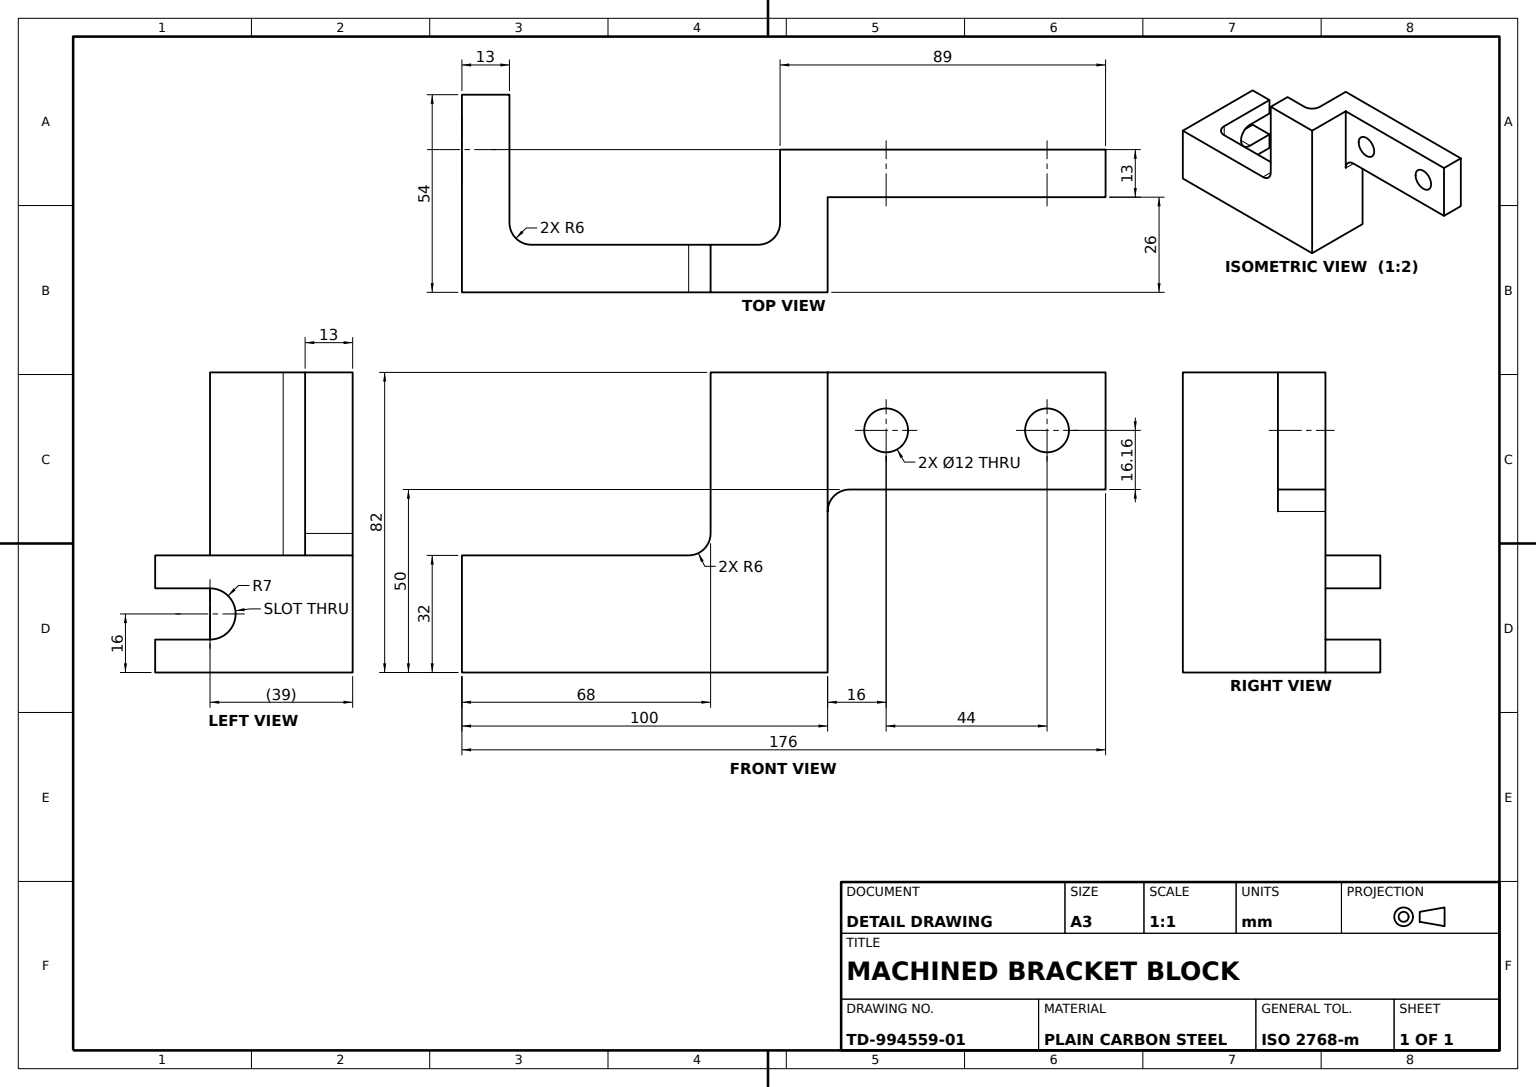
SolidWorks part; units mm, degrees
material "Plain Carbon Steel"
ref_plane "Front Plane" through (0, 0, 0) normal (0, 0, 1) x (1, 0, 0)
ref_plane "Top Plane" through (0, 0, 0) normal (0, 1, 0) x (1, 0, 0)
ref_plane "Right Plane" through (0, 0, 0) normal (1, 0, 0) x (0, 0, -1)
sketch "Base Profile Sketch" plane through (0, 0, 0) normal (0, 0, 1) x (1, 0, 0)
  line L0 (0, 0) -> (100, 0)
  line L1 (100, 0) -> (100, 82)
  line L2 (100, 82) -> (68, 82)
  line L3 (68, 82) -> (68, 38)
  line L4 (62, 32) -> (0, 32)
  line L5 (0, 32) -> (0, 0)
  arc A0 (62, 32) -> (68, 38) centre (62, 38) ccw
  dimension "D1" = 6
  dimension "D2" = 68
  dimension "D3" = 100
  dimension "D4" = 82
extrude "Base Profile 13mm" add sketch "Base Profile Sketch" along normal blind 13
sketch "Upright Block Sketch" plane through (0, 0, 0) normal (0, -1, 0) x (1, 0, 0)
  line L0 (0, 0) -> (0, -54)
  line L1 (0, -54) -> (13, -54)
  line L2 (13, -54) -> (13, -6)
  line L3 (0, 0) -> (100, 0) construction
  line L5 (87, -6) -> (87, -26)
  line L6 (87, -26) -> (100, -26)
  line L7 (100, -26) -> (100, 0)
  line L8 (19, 0) -> (81, 0)
  line L9 (0, 0) -> (100, 0)
  line L10 (100, 13) -> (100, 0) construction
  arc A0 (19, 0) -> (13, -6) centre (19, -6) ccw
  arc A1 (81, 0) -> (87, -6) centre (81, -6) cw
  point P14 (13, 0)
  line M1 (0, 0) -> (100, 0)
  dimension "D1" = 6
  dimension "D2" = 6
  dimension "D3" = 13
  dimension "D4" = 26
  dimension "D5" = 54
extrude "Upright Block 82mm" add sketch "Upright Block Sketch" against normal blind 82 contours A0 L0 L1 L2 M1 | A1 L5 L6 L7 M1
sketch "Rectangular Cut Sketch" plane through (0, 0, 0) normal (-1, 0, 0) x (0, 0, 1)
  line L0 (-54, 82) -> (0, 82)
  line L1 (0, 82) -> (0, 32)
  line L2 (0, 38) -> (0, 32) construction
  line L3 (0, 82) -> (0, 32) construction
  line L4 (0, 32) -> (-54, 32)
  line L5 (-54, 82) -> (-54, 0) construction
  line L6 (-54, 32) -> (-54, 82)
  dimension "D1" = 50
extrude "Rectangular Cut 20mm" cut sketch "Rectangular Cut Sketch" against normal blind 20
sketch "Pocket Cut Sketch" plane through (0, 0, -54) normal (0, 0, -1) x (-1, 0, 0)
  line L0 (-13, 32) -> (0, 32)
  line L1 (0, 32) -> (0, 0)
  line L2 (0, 0) -> (-13, 0)
  line L3 (-13, 0) -> (-13, 32)
extrude "Pocket Cut 13mm" cut sketch "Pocket Cut Sketch" against normal blind 13
sketch "Slot Cut Sketch" plane through (0, 0, 0) normal (-1, 0, 0) x (0, 0, 1)
  line L0 (13, 32) -> (-41, 32) construction
  line L1 (-41, 0) -> (-41, 32) construction
  line L2 (-41, 9) -> (-26, 9)
  line L4 (-26, 23) -> (-41, 23)
  line L6 (-41, 23) -> (-41, 9)
  arc A0 (-26, 9) -> (-26, 23) centre (-26, 16) ccw
  dimension "D1" = 14
  dimension "D2" = 7
  dimension "D3" = 39
  dimension "D4" = 16
extrude "Slot Cut 14mm" cut sketch "Slot Cut Sketch" against normal blind 13
sketch "Mounting Flange Sketch" plane through (0, 0, -26) normal (0, 0, -1) x (-1, 0, 0)
  line L0 (-100, 82) -> (-176, 82)
  line L1 (-176, 82) -> (-176, 50)
  line L2 (-176, 50) -> (-106, 50)
  line L3 (-100, 82) -> (-100, 0) construction
  line L4 (-100, 82) -> (-100, 44)
  line L5 (-87, 82) -> (-87, 0) construction
  line L6 (-87, 0) -> (-100, 0) construction
  arc A0 (-106, 50) -> (-100, 44) centre (-106, 44) cw
  point P11 (-100, 50)
  dimension "D1" = 6
  dimension "D2" = 89
  dimension "D3" = 50
extrude "Mounting Flange 6mm" add sketch "Mounting Flange Sketch" against normal blind 13
sketch "Flange Holes Sketch" plane through (0, 0, -13) normal (0, 0, 1) x (1, 0, 0)
  line L0 (176, 82) -> (176, 50) construction
  line L2 (176, 50) -> (106, 50) construction
  circle A0 centre (116, 66.1569) radius 6
  circle A1 centre (160, 66.1569) radius 6
  dimension "D1" = 12
  dimension "D2" = 12
  dimension "D5" = 12
  dimension "D3" = 16
  dimension "D4" = 44
  dimension "D6" = 16.1569
extrude "Flange Holes 2xØ12" cut sketch "Flange Holes Sketch" against normal blind 13
